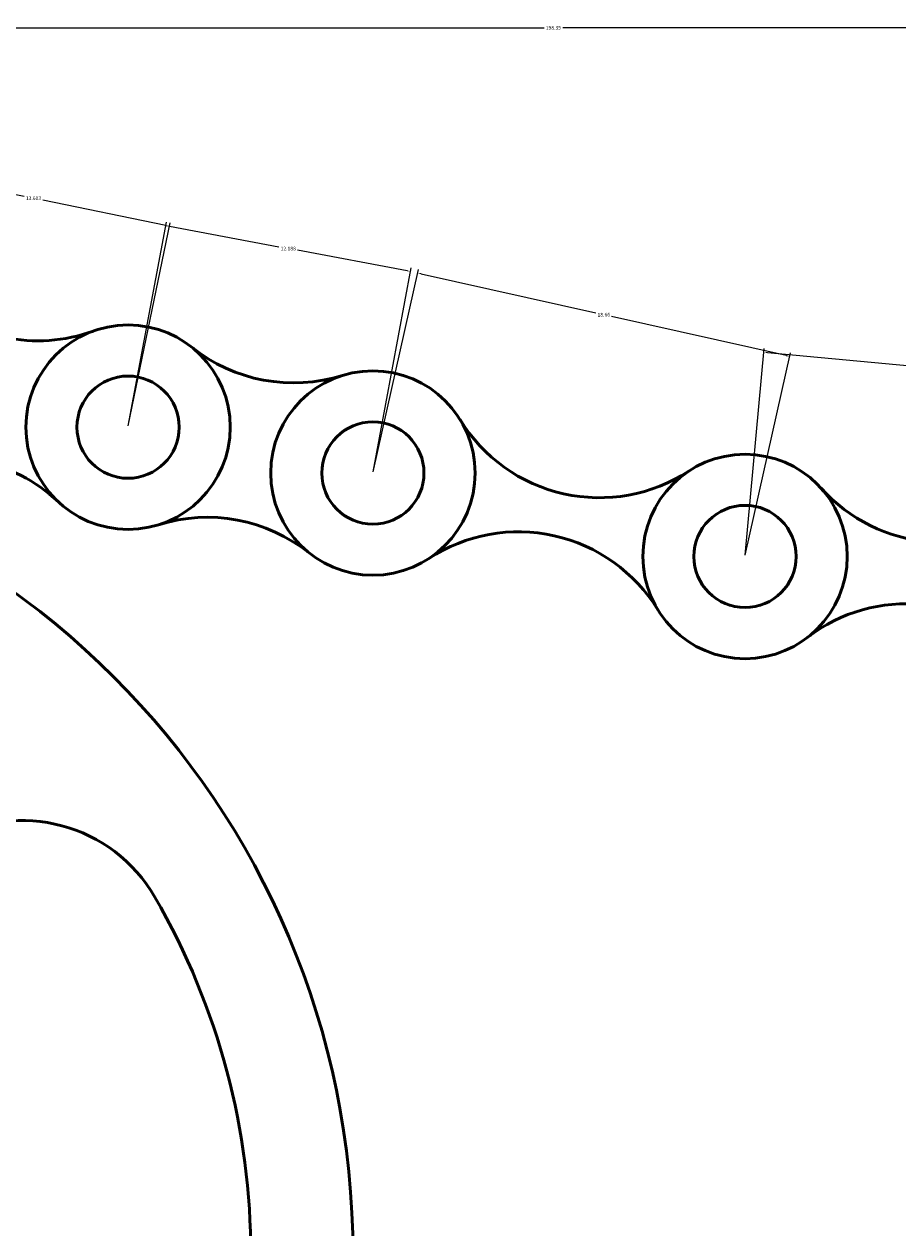
# Model space of a CAD drawing. Units: inches. Extents: x 413 to 622, y 326 to 447.
# Tile 9 of 15: x 497 to 539, y 388 to 447. Entities that reach past the tile are written whole.
import ezdxf

# ---------------------------------------------------------------- set-up
doc = ezdxf.new("R2010")
doc.units = ezdxf.units.IN
doc.header["$MEASUREMENT"] = 0
doc.layers.add('M-DIMS', color=2, linetype='Continuous', lineweight=18)
doc.layers.add('M-OUTL', color=7, linetype='Continuous', lineweight=50)
doc.styles.get("Standard").update_dxf_attribs({"font": 'arial.ttf'})
doc.dimstyles.get("Standard").update_dxf_attribs({"dimtxt": 0.18, "dimasz": 0.18, "dimexe": 0.18, "dimexo": 0.0625, "dimgap": 0.09, "dimtad": 0, "dimtih": 1, "dimtoh": 1, "dimdec": 4, "dimzin": 0, "dimdsep": 46, "dimtxsty": 'Standard', "dimcen": 0.09, "dimadec": 0, "dimazin": 0, "dimtfac": 1, "dimtdec": 4, "dimtofl": 0, "dimtmove": 0, "dimatfit": 3, "dimfxl": 1, "dimtolj": 1, "dimtzin": 0, "dimarcsym": 0})

# ---------------------------------------------------------------- blocks, each defined once
blk = doc.blocks.new('CHAIN-ROLLER-PIN')
for radius in [5, 2.5]:
    blk.add_circle((5, 5), radius)
blk = doc.blocks.new('SPROCKET-WEB-SLOT')
for centre, radius, start, end in [((31.317, 35), 35, 210, 270), ((31.317, 7.5), 7.5, 270, 90)]:
    blk.add_arc(centre, radius, start, end)
blk = doc.blocks.new('CHAIN-LINK-WAIST-P13_603')
for centre, start, end in [((7.205, 15.87), 226.77186, 289.86266), ((2.718, -5.829), 46.77186, 109.86266)]:
    blk.add_arc(centre, 8, start, end)
blk = doc.blocks.new('CHAIN-LINK-WAIST-P12_188')
for centre, start, end in [((6.613, 16.319), 231.4363, 287.34282), ((2.384, -6.255), 51.4363, 107.34282)]:
    blk.add_arc(centre, 8, start, end)
blk = doc.blocks.new('CHAIN-LINK-WAIST-P18_660')
for centre, start, end in [((8.344, 13.487), 211.50374, 303.22962), ((4.384, -4.18), 31.50374, 123.22962)]:
    blk.add_arc(centre, 8, start, end)
blk = doc.blocks.new('CHAIN-LINK-WAIST-P17_664')
for centre, start, end in [((6.624, 13.651), 221.93853, 307.52912), ((4.873, -5.347), 41.93853, 127.52912)]:
    blk.add_arc(centre, 8, start, end)
blk = doc.blocks.new('*D11')
at = {"layer": 'Defpoints', "color": 0, "transparency": 16777216}
for p in [(621.66, 446.422), (621.66, 388.074), (423.314, 378.888)]:
    blk.add_point(p, dxfattribs=at)
at = {"layer": 'M-DIMS', "color": 0, "lineweight": -2, "transparency": 16777216}
for p, q in [((423.314, 378.95), (423.314, 446.602)), ((423.494, 446.422), (522.031, 446.422)), ((621.48, 446.422), (522.943, 446.422)), ((621.66, 388.137), (621.66, 446.602))]:
    blk.add_line(p, q, dxfattribs=at)
at = {"layer": 'M-DIMS', "color": 0, "transparency": 16777216}
for points in [[(423.494, 446.452), (423.494, 446.392), (423.314, 446.422)], [(621.48, 446.452), (621.48, 446.392), (621.66, 446.422)]]:
    blk.add_solid(points, dxfattribs=at)
at = {"layer": 'M-DIMS', "color": 0, "transparency": 16777216, "insert": (522.487, 446.422), "char_height": 0.18, "attachment_point": 5}
blk.add_mtext('\\A1;198.35', dxfattribs=at)
blk = doc.blocks.new('*D17')
at = {"layer": 'Defpoints', "color": 0, "transparency": 16777216}
for p in [(503.707, 436.707), (488.355, 429.638), (501.676, 426.884)]:
    blk.add_point(p, dxfattribs=at)
at = {"layer": 'M-DIMS', "color": 0, "lineweight": -2, "transparency": 16777216}
for p, q in [((488.368, 429.7), (490.423, 439.637)), ((490.563, 439.425), (496.592, 438.178)), ((503.531, 436.743), (497.502, 437.99)), ((501.689, 426.945), (503.744, 436.883))]:
    blk.add_line(p, q, dxfattribs=at)
at = {"layer": 'M-DIMS', "color": 0, "transparency": 16777216}
for points in [[(490.569, 439.454), (490.557, 439.395), (490.386, 439.461)], [(503.537, 436.772), (503.525, 436.714), (503.707, 436.707)]]:
    blk.add_solid(points, dxfattribs=at)
at = {"layer": 'M-DIMS', "color": 0, "transparency": 16777216, "insert": (497.047, 438.084), "char_height": 0.18, "attachment_point": 5}
blk.add_mtext('\\A1;13.603', dxfattribs=at)
blk = doc.blocks.new('*D18')
at = {"layer": 'Defpoints', "color": 0, "transparency": 16777216}
for p in [(515.502, 434.499), (501.676, 426.884), (513.655, 424.64)]:
    blk.add_point(p, dxfattribs=at)
at = {"layer": 'M-DIMS', "color": 0, "lineweight": -2, "transparency": 16777216}
for p, q in [((501.688, 426.945), (503.556, 436.92)), ((503.7, 436.71), (509.057, 435.706)), ((515.325, 434.532), (509.968, 435.536)), ((513.667, 424.701), (515.535, 434.676))]:
    blk.add_line(p, q, dxfattribs=at)
at = {"layer": 'M-DIMS', "color": 0, "transparency": 16777216}
for points in [[(503.705, 436.739), (503.694, 436.68), (503.523, 436.743)], [(515.331, 434.561), (515.32, 434.502), (515.502, 434.499)]]:
    blk.add_solid(points, dxfattribs=at)
at = {"layer": 'M-DIMS', "color": 0, "transparency": 16777216, "insert": (509.513, 435.621), "char_height": 0.18, "attachment_point": 5}
blk.add_mtext('\\A1;12.188', dxfattribs=at)
blk = doc.blocks.new('*D19')
at = {"layer": 'Defpoints', "color": 0, "transparency": 16777216}
for p in [(534.057, 430.346), (513.655, 424.64), (531.863, 420.559)]:
    blk.add_point(p, dxfattribs=at)
at = {"layer": 'M-DIMS', "color": 0, "lineweight": -2, "transparency": 16777216}
for p, q in [((513.669, 424.701), (515.888, 434.603)), ((516.025, 434.388), (524.568, 432.473)), ((533.881, 430.386), (525.338, 432.301)), ((531.877, 420.62), (534.096, 430.522))]:
    blk.add_line(p, q, dxfattribs=at)
at = {"layer": 'M-DIMS', "color": 0, "transparency": 16777216}
for points in [[(516.031, 434.417), (516.018, 434.359), (515.849, 434.427)], [(533.888, 430.415), (533.875, 430.357), (534.057, 430.346)]]:
    blk.add_solid(points, dxfattribs=at)
at = {"layer": 'M-DIMS', "color": 0, "transparency": 16777216, "insert": (524.953, 432.387), "char_height": 0.18, "attachment_point": 5}
blk.add_mtext('\\A1;18.66', dxfattribs=at)
blk = doc.blocks.new('*D20')
at = {"layer": 'Defpoints', "color": 0, "transparency": 16777216}
for p in [(550.373, 428.926), (531.863, 420.559), (549.452, 418.938)]:
    blk.add_point(p, dxfattribs=at)
at = {"layer": 'M-DIMS', "color": 0, "lineweight": -2, "transparency": 16777216}
for p, q in [((531.869, 420.621), (532.8, 430.726)), ((532.963, 430.53), (541.124, 429.778)), ((550.194, 428.942), (542.033, 429.694)), ((549.458, 419), (550.39, 429.105))]:
    blk.add_line(p, q, dxfattribs=at)
at = {"layer": 'M-DIMS', "color": 0, "transparency": 16777216}
for points in [[(532.966, 430.56), (532.96, 430.501), (532.784, 430.547)], [(550.197, 428.972), (550.191, 428.912), (550.373, 428.926)]]:
    blk.add_solid(points, dxfattribs=at)
at = {"layer": 'M-DIMS', "color": 0, "transparency": 16777216, "insert": (541.578, 429.736), "char_height": 0.18, "attachment_point": 5}
blk.add_mtext('\\A1;17.664', dxfattribs=at)

msp = doc.modelspace()

# ---------------------------------------------------------------- linework, layer by layer
at = {"layer": 'M-OUTL'}
msp.add_circle((472.6836, 386.3915), 40, dxfattribs=at)

# ---------------------------------------------------------------- block references
for name, p in [('CHAIN-LINK-WAIST-P13_603', (490.054, 423.241)), ('CHAIN-ROLLER-PIN', (496.6765, 421.8844)), ('CHAIN-LINK-WAIST-P12_188', (503.167, 420.73)), ('CHAIN-ROLLER-PIN', (508.6556, 419.6403)), ('CHAIN-LINK-WAIST-P18_660', (516.395, 417.946)), ('CHAIN-ROLLER-PIN', (526.8634, 415.5593)), ('CHAIN-LINK-WAIST-P17_664', (534.909, 415.596))]:
    msp.add_blockref(name, p, dxfattribs=at)
at = {"layer": 'M-OUTL', "rotation": 119.9999999999996}
msp.add_blockref('SPROCKET-WEB-SLOT', (518.6523, 376.7703), dxfattribs=at)

# ---------------------------------------------------------------- dimensions: what is measured, and where the dimension line sits
at = {"layer": 'M-DIMS'}
dim = msp.add_linear_dim(base=(621.66, 446.422), p1=(423.3136, 378.8878), p2=(621.66, 388.0741), dimstyle='Standard', override={"dimdec": 2, "dimlfac": 1, "dimrnd": 0, "dimzin": 0, "dimdsep": 46, "dimlunit": 2}, dxfattribs=at)
dim.commit()
dim.dimension.update_dxf_attribs({"geometry": '*D11', "text_midpoint": (522.4868, 446.422)})
for base, p1, p2, angle, override, picture, middle in [((503.7072, 436.7066), (488.3553, 429.6383), (501.6761, 426.8839), 348.317261, {"dimdec": 3, "dimlfac": 1, "dimrnd": 0, "dimzin": 0, "dimdsep": 46, "dimlunit": 2}, '*D17', (497.0468, 438.0838)), ((515.50213, 434.49881), (501.67606, 426.88391), (513.65521, 424.63981), 349.389559, {"dimdec": 3, "dimlfac": 1, "dimrnd": 0, "dimzin": 0, "dimdsep": 46, "dimlunit": 2}, '*D18', (509.51255, 435.62086)), ((534.0568, 430.3464), (513.6552, 424.6398), (531.863, 420.5588), 347.366684, {"dimdec": 2, "dimlfac": 1, "dimrnd": 0, "dimzin": 0, "dimdsep": 46, "dimlunit": 2}, '*D19', (524.9529, 432.3869)), ((550.373, 428.9257), (531.863, 420.5588), (549.4524, 418.9375), 354.733826, {"dimdec": 3, "dimlfac": 1, "dimrnd": 0, "dimzin": 0, "dimdsep": 46, "dimlunit": 2}, '*D20', (541.5783, 429.7363))]:
    dim = msp.add_linear_dim(base=base, p1=p1, p2=p2, angle=angle, dimstyle='Standard', override=override, dxfattribs=at)
    dim.commit()
    dim.dimension.update_dxf_attribs({"geometry": picture, "text_midpoint": middle})

doc.saveas('drawing.dxf')
